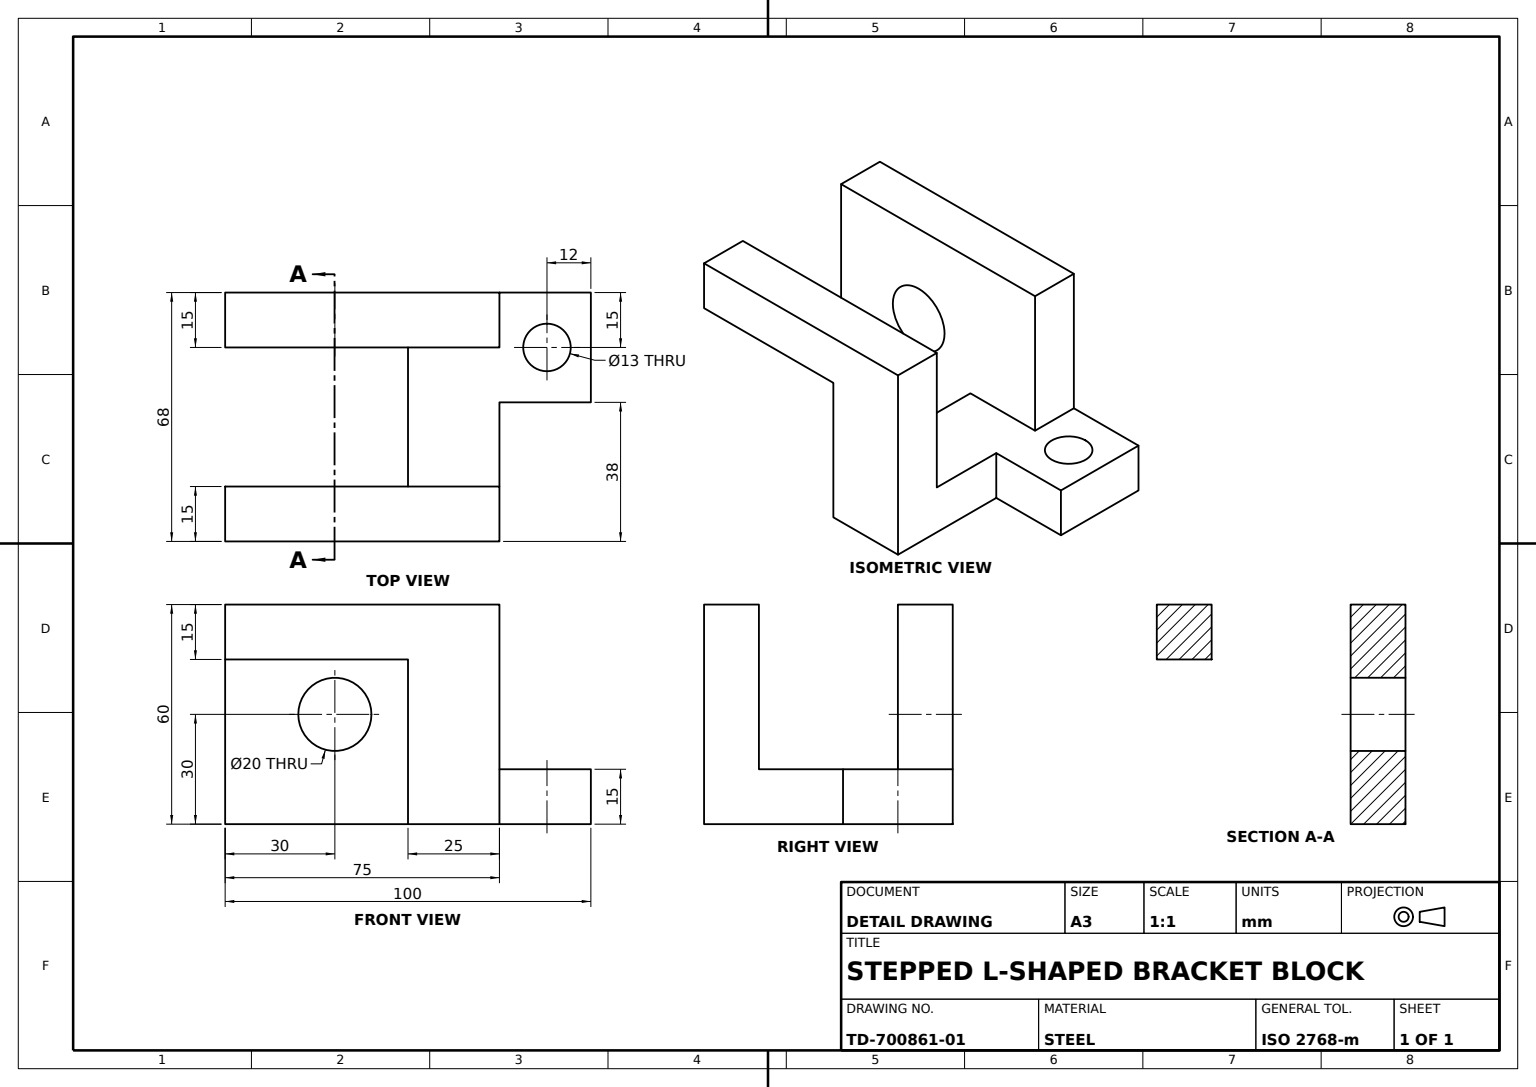
from build123d import *

# Parameters (mm, degrees)
L_SIDE_WALL_DEPTH            = 15
BASE_FLANGE_WITH_TAB_DEPTH   = 15
UPRIGHT_PLATE_SKETCH_W       = 75
UPRIGHT_PLATE_SKETCH_H       = 15
UPRIGHT_PLATE_DEPTH          = 60
UPRIGHT_CROSS_HOLE_SKETCH_R  = 10
UPRIGHT_CROSS_HOLE_DEPTH     = 118.68177429
TAB_MOUNTING_HOLE_DEPTH      = 111.788086002
TAB_MOUNTING_HOLE_DEPTH_BACK = 111.788086002
TAB_MOUNTING_HOLE_SKETCH_R   = 6.5


with BuildPart() as part:
    # L Side Wall Sketch → L Side Wall (new body)
    with BuildSketch(Plane.XY):
        Polygon((0, 0), (0, 60), (-75, 60), (-75, 45), (-25, 45), (-25, 0), align=None)
    extrude(amount=-L_SIDE_WALL_DEPTH)

    # Base Flange Sketch → Base Flange With Tab (add)
    with BuildSketch(Plane(origin=(0, 0, 0), x_dir=(1, 0, 0), z_dir=(0, 1, 0))):
        Polygon((25, 68), (25, 38), (0, 38), (0, 0), (-25, 0), (-25, 53), (0, 53), (0, 68), align=None)
    extrude(amount=BASE_FLANGE_WITH_TAB_DEPTH)

    # Upright Plate Sketch → Upright Plate (add)
    with BuildSketch(Plane(origin=(0, 0, 0), x_dir=(1, 0, 0), z_dir=(0, 1, 0))):
        with Locations((-37.5, 60.5)):
            Rectangle(UPRIGHT_PLATE_SKETCH_W, UPRIGHT_PLATE_SKETCH_H)
    extrude(amount=UPRIGHT_PLATE_DEPTH)

    # Upright Cross Hole Sketch → Upright Cross Hole (cut, through all)
    with BuildSketch(Plane(origin=(0, 0, -68), x_dir=(-1, 0, 0), z_dir=(0, 0, -1))):
        with Locations((45, 30)):
            Circle(UPRIGHT_CROSS_HOLE_SKETCH_R)
    extrude(amount=-UPRIGHT_CROSS_HOLE_DEPTH, mode=Mode.SUBTRACT)

    # Tab Mounting Hole Sketch → Tab Mounting Hole (cut, two sides: drawn at the far end of the back side and taken through both)
    with BuildSketch(Plane(origin=(0, 15, 0), x_dir=(1, 0, 0), z_dir=(0, 1, 0)).offset(-TAB_MOUNTING_HOLE_DEPTH_BACK)):
        with Locations(Location((13, 53, 0), (0, 0, 270))):
            Circle(TAB_MOUNTING_HOLE_SKETCH_R)
    extrude(amount=TAB_MOUNTING_HOLE_DEPTH + TAB_MOUNTING_HOLE_DEPTH_BACK, mode=Mode.SUBTRACT)


solid = part.part
